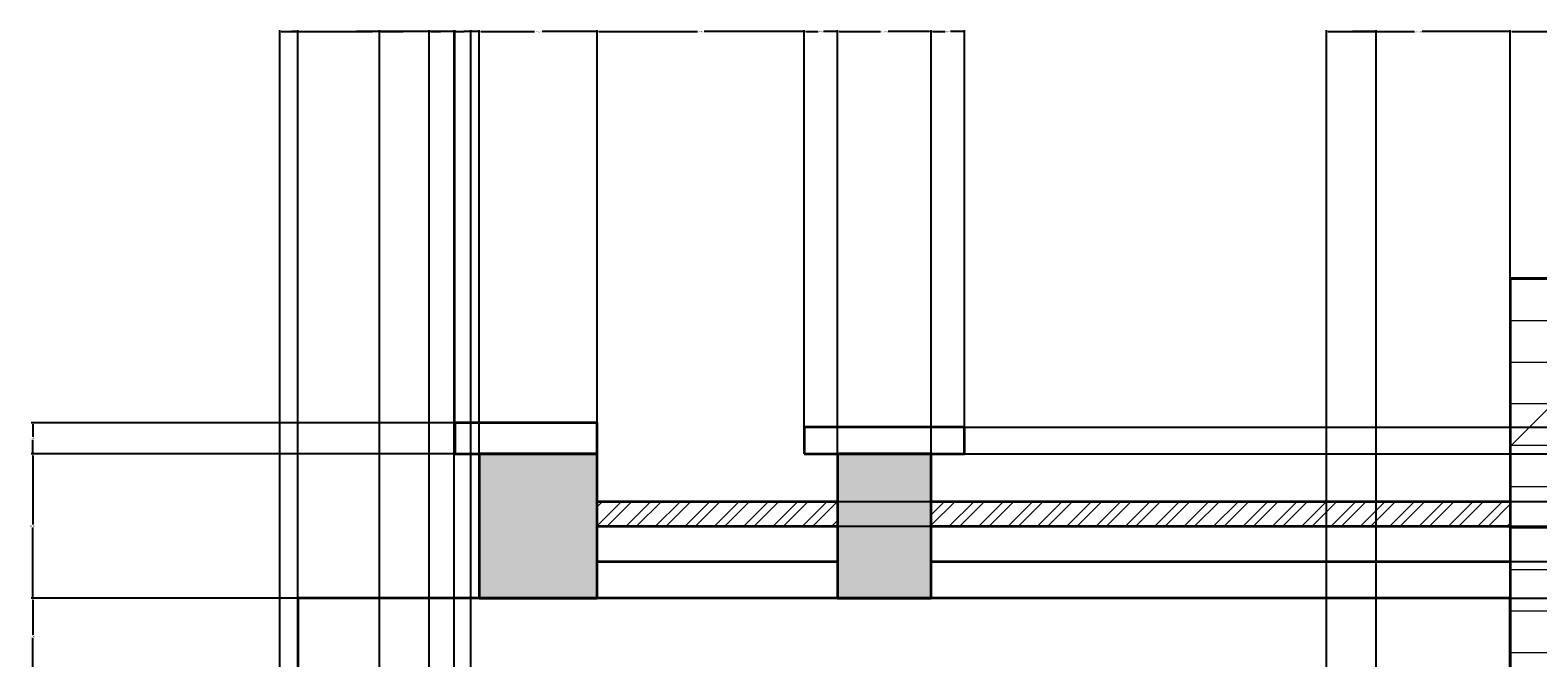
# Model space of a CAD drawing. Units: inches. Extents: x -13 to 630, y -103 to 275.
# Tile 5 of 9: x -13 to 168, y 199 to 275. Entities that reach past the tile are written whole.
import ezdxf

# ---------------------------------------------------------------- set-up
doc = ezdxf.new("R2010")
doc.units = ezdxf.units.IN
doc.header["$MEASUREMENT"] = 0
for name, color, linetype, lineweight in [('A-ANNO-DIMS', 2, 'Continuous', 18), ('A-ELEV', 7, 'Continuous', 35), ('A-ELEV-PATT', 8, 'Continuous', 13)]:
    doc.layers.add(name, color=color, linetype=linetype, lineweight=lineweight)
doc.styles.get("Standard").update_dxf_attribs({"font": 'arial.ttf'})
doc.dimstyles.get("Standard").update_dxf_attribs({"dimtxt": 0.18, "dimasz": 0.18, "dimexe": 0.18, "dimexo": 0.0625, "dimgap": 0.09, "dimtad": 0, "dimtih": 1, "dimtoh": 1, "dimdec": 4, "dimzin": 0, "dimdsep": 46, "dimtxsty": 'Standard', "dimcen": 0.09, "dimadec": 0, "dimazin": 0, "dimtfac": 1, "dimtdec": 4, "dimtofl": 0, "dimtmove": 0, "dimatfit": 3, "dimfxl": 1, "dimtolj": 1, "dimtzin": 0, "dimarcsym": 0})

# ---------------------------------------------------------------- blocks, each defined once
blk = doc.blocks.new('*D7')
at = {"layer": 'A-ANNO-DIMS', "color": 0, "lineweight": -2, "transparency": 16777216}
for p, q in [((16.71, 5.14), (16.71, 275.01)), ((16.89, 274.83), (25.5, 274.83)), ((34.53, 274.83), (25.92, 274.83)), ((34.71, 5.14), (34.71, 275.01))]:
    blk.add_line(p, q, dxfattribs=at)
at = {"layer": 'A-ANNO-DIMS', "color": 0, "transparency": 16777216}
for points in [[(16.89, 274.86), (16.89, 274.8), (16.71, 274.83)], [(34.53, 274.86), (34.53, 274.8), (34.71, 274.83)]]:
    blk.add_solid(points, dxfattribs=at)
at = {"layer": 'Defpoints', "color": 0, "transparency": 16777216}
for p in [(34.71, 274.83), (16.71, 5.08), (34.71, 5.08)]:
    blk.add_point(p, dxfattribs=at)
at = {"layer": 'A-ANNO-DIMS', "color": 0, "transparency": 16777216, "insert": (25.71, 274.83), "char_height": 0.18, "attachment_point": 5}
blk.add_mtext('\\A1;18', dxfattribs=at)
blk = doc.blocks.new('*D8')
at = {"layer": 'A-ANNO-DIMS', "color": 0, "lineweight": -2, "transparency": 16777216}
for p, q in [((142.71, 5.14), (142.71, 275.01)), ((142.89, 274.83), (153.31, 274.83)), ((164.66, 274.83), (154.24, 274.83)), ((164.84, 5.14), (164.84, 275.01))]:
    blk.add_line(p, q, dxfattribs=at)
at = {"layer": 'A-ANNO-DIMS', "color": 0, "transparency": 16777216}
for points in [[(142.89, 274.86), (142.89, 274.8), (142.71, 274.83)], [(164.66, 274.86), (164.66, 274.8), (164.84, 274.83)]]:
    blk.add_solid(points, dxfattribs=at)
at = {"layer": 'Defpoints', "color": 0, "transparency": 16777216}
for p in [(164.84, 274.83), (142.71, 5.08), (164.84, 5.08)]:
    blk.add_point(p, dxfattribs=at)
at = {"layer": 'A-ANNO-DIMS', "color": 0, "transparency": 16777216, "insert": (153.78, 274.83), "char_height": 0.18, "attachment_point": 5}
blk.add_mtext('\\A1;22.133', dxfattribs=at)
blk = doc.blocks.new('*D27')
at = {"layer": 'A-ANNO-DIMS', "color": 0, "lineweight": -2, "transparency": 16777216}
for p, q in [((164.84, 245.14), (164.84, 275.01)), ((165.02, 274.83), (254.62, 274.83)), ((345.13, 274.83), (255.53, 274.83)), ((345.31, 245.14), (345.31, 275.01))]:
    blk.add_line(p, q, dxfattribs=at)
at = {"layer": 'A-ANNO-DIMS', "color": 0, "transparency": 16777216}
for points in [[(165.02, 274.86), (165.02, 274.8), (164.84, 274.83)], [(345.13, 274.86), (345.13, 274.8), (345.31, 274.83)]]:
    blk.add_solid(points, dxfattribs=at)
at = {"layer": 'Defpoints', "color": 0, "transparency": 16777216}
for p in [(345.31, 274.83), (164.84, 245.08), (345.31, 245.08)]:
    blk.add_point(p, dxfattribs=at)
at = {"layer": 'A-ANNO-DIMS', "color": 0, "transparency": 16777216, "insert": (255.08, 274.83), "char_height": 0.18, "attachment_point": 5}
blk.add_mtext('\\A1;180.46', dxfattribs=at)
blk = doc.blocks.new('*D30')
at = {"layer": 'A-ANNO-DIMS', "color": 0, "lineweight": -2, "transparency": 16777216}
for p, q in [((164.84, 245.14), (164.84, 275.01)), ((165.02, 274.83), (170.63, 274.83)), ((176.66, 274.83), (171.05, 274.83)), ((176.84, 233.14), (176.84, 275.01))]:
    blk.add_line(p, q, dxfattribs=at)
at = {"layer": 'A-ANNO-DIMS', "color": 0, "transparency": 16777216}
for points in [[(165.02, 274.86), (165.02, 274.8), (164.84, 274.83)], [(176.66, 274.86), (176.66, 274.8), (176.84, 274.83)]]:
    blk.add_solid(points, dxfattribs=at)
at = {"layer": 'Defpoints', "color": 0, "transparency": 16777216}
for p in [(176.84, 274.83), (164.84, 245.08), (176.84, 233.08)]:
    blk.add_point(p, dxfattribs=at)
at = {"layer": 'A-ANNO-DIMS', "color": 0, "transparency": 16777216, "insert": (170.84, 274.83), "char_height": 0.18, "attachment_point": 5}
blk.add_mtext('\\A1;12', dxfattribs=at)
blk = doc.blocks.new('*D67')
at = {"layer": 'A-ANNO-DIMS', "color": 0, "lineweight": -2, "transparency": 16777216}
for p, q in [((28.71, 113.14), (28.71, 275.01)), ((28.89, 274.83), (31.56, 274.83)), ((34.53, 274.83), (31.86, 274.83)), ((34.71, 107.14), (34.71, 275.01))]:
    blk.add_line(p, q, dxfattribs=at)
at = {"layer": 'A-ANNO-DIMS', "color": 0, "transparency": 16777216}
for points in [[(28.89, 274.86), (28.89, 274.8), (28.71, 274.83)], [(34.53, 274.86), (34.53, 274.8), (34.71, 274.83)]]:
    blk.add_solid(points, dxfattribs=at)
at = {"layer": 'Defpoints', "color": 0, "transparency": 16777216}
for p in [(34.71, 274.83), (28.71, 113.08), (34.71, 107.08)]:
    blk.add_point(p, dxfattribs=at)
at = {"layer": 'A-ANNO-DIMS', "color": 0, "transparency": 16777216, "insert": (31.71, 274.83), "char_height": 0.18, "attachment_point": 5}
blk.add_mtext('\\A1;6', dxfattribs=at)
blk = doc.blocks.new('*D68')
at = {"layer": 'A-ANNO-DIMS', "color": 0, "lineweight": -2, "transparency": 16777216}
for p, q in [((34.71, 107.14), (34.71, 275.01)), ((34.89, 274.83), (36.06, 274.83)), ((37.53, 274.83), (36.36, 274.83)), ((37.71, 104.14), (37.71, 275.01))]:
    blk.add_line(p, q, dxfattribs=at)
at = {"layer": 'A-ANNO-DIMS', "color": 0, "transparency": 16777216}
for points in [[(34.89, 274.86), (34.89, 274.8), (34.71, 274.83)], [(37.53, 274.86), (37.53, 274.8), (37.71, 274.83)]]:
    blk.add_solid(points, dxfattribs=at)
at = {"layer": 'Defpoints', "color": 0, "transparency": 16777216}
for p in [(37.71, 274.83), (34.71, 107.08), (37.71, 104.08)]:
    blk.add_point(p, dxfattribs=at)
at = {"layer": 'A-ANNO-DIMS', "color": 0, "transparency": 16777216, "insert": (36.21, 274.83), "char_height": 0.18, "attachment_point": 5}
blk.add_mtext('\\A1;3', dxfattribs=at)
blk = doc.blocks.new('*D69')
at = {"layer": 'A-ANNO-DIMS', "color": 0, "lineweight": -2, "transparency": 16777216}
for p, q in [((37.71, 104.14), (37.71, 275.01)), ((37.89, 274.83), (38.56, 274.83)), ((39.53, 274.83), (38.86, 274.83)), ((39.71, 102.14), (39.71, 275.01))]:
    blk.add_line(p, q, dxfattribs=at)
at = {"layer": 'A-ANNO-DIMS', "color": 0, "transparency": 16777216}
for points in [[(37.89, 274.86), (37.89, 274.8), (37.71, 274.83)], [(39.53, 274.86), (39.53, 274.8), (39.71, 274.83)]]:
    blk.add_solid(points, dxfattribs=at)
at = {"layer": 'Defpoints', "color": 0, "transparency": 16777216}
for p in [(39.71, 274.83), (37.71, 104.08), (39.71, 102.08)]:
    blk.add_point(p, dxfattribs=at)
at = {"layer": 'A-ANNO-DIMS', "color": 0, "transparency": 16777216, "insert": (38.71, 274.83), "char_height": 0.18, "attachment_point": 5}
blk.add_mtext('\\A1;2', dxfattribs=at)
blk = doc.blocks.new('*D70')
at = {"layer": 'A-ANNO-DIMS', "color": 0, "lineweight": -2, "transparency": 16777216}
for p, q in [((142.71, 107.14), (142.71, 275.01)), ((142.89, 274.83), (145.56, 274.83)), ((148.53, 274.83), (145.86, 274.83)), ((148.71, 113.14), (148.71, 275.01))]:
    blk.add_line(p, q, dxfattribs=at)
at = {"layer": 'A-ANNO-DIMS', "color": 0, "transparency": 16777216}
for points in [[(142.89, 274.86), (142.89, 274.8), (142.71, 274.83)], [(148.53, 274.86), (148.53, 274.8), (148.71, 274.83)]]:
    blk.add_solid(points, dxfattribs=at)
at = {"layer": 'Defpoints', "color": 0, "transparency": 16777216}
for p in [(148.71, 274.83), (148.71, 113.08), (142.71, 107.08)]:
    blk.add_point(p, dxfattribs=at)
at = {"layer": 'A-ANNO-DIMS', "color": 0, "transparency": 16777216, "insert": (145.71, 274.83), "char_height": 0.18, "attachment_point": 5}
blk.add_mtext('\\A1;6', dxfattribs=at)
blk = doc.blocks.new('*D88')
at = {"layer": 'A-ANNO-DIMS', "color": 0, "lineweight": -2, "transparency": 16777216}
for p, q in [((18.81, 206.53), (-13.22, 206.53)), ((-13.04, 206.35), (-13.04, 202.11)), ((-13.04, 197.5), (-13.04, 201.74)), ((18.81, 197.32), (-13.22, 197.32))]:
    blk.add_line(p, q, dxfattribs=at)
at = {"layer": 'A-ANNO-DIMS', "color": 0, "transparency": 16777216}
for points in [[(-13.07, 206.35), (-13.01, 206.35), (-13.04, 206.53)], [(-13.07, 197.5), (-13.01, 197.5), (-13.04, 197.32)]]:
    blk.add_solid(points, dxfattribs=at)
at = {"layer": 'Defpoints', "color": 0, "transparency": 16777216}
for p in [(-13.04, 206.53), (18.87, 206.53), (18.87, 197.32)]:
    blk.add_point(p, dxfattribs=at)
at = {"layer": 'A-ANNO-DIMS', "color": 0, "transparency": 16777216, "insert": (-13.04, 201.92), "char_height": 0.18, "attachment_point": 5}
blk.add_mtext('\\A1;9.206', dxfattribs=at)
blk = doc.blocks.new('*D89')
at = {"layer": 'A-ANNO-DIMS', "color": 0, "lineweight": -2, "transparency": 16777216}
for p, q in [((95.18, 210.97), (630.03, 210.97)), ((629.85, 210.79), (629.85, 208.93)), ((629.85, 206.71), (629.85, 208.57)), ((95.18, 206.53), (630.03, 206.53))]:
    blk.add_line(p, q, dxfattribs=at)
at = {"layer": 'A-ANNO-DIMS', "color": 0, "transparency": 16777216}
for points in [[(629.82, 210.79), (629.88, 210.79), (629.85, 210.97)], [(629.82, 206.71), (629.88, 206.71), (629.85, 206.53)]]:
    blk.add_solid(points, dxfattribs=at)
at = {"layer": 'Defpoints', "color": 0, "transparency": 16777216}
for p in [(95.12, 210.97), (629.85, 210.97), (95.12, 206.53)]:
    blk.add_point(p, dxfattribs=at)
at = {"layer": 'A-ANNO-DIMS', "color": 0, "transparency": 16777216, "insert": (629.85, 208.75), "char_height": 0.18, "attachment_point": 5}
blk.add_mtext('\\A1;4.442', dxfattribs=at)
blk = doc.blocks.new('*D90')
at = {"layer": 'A-ANNO-DIMS', "color": 0, "lineweight": -2, "transparency": 16777216}
for p, q in [((95.18, 218.21), (630.03, 218.21)), ((629.85, 218.03), (629.85, 214.77)), ((629.85, 211.15), (629.85, 214.41)), ((95.18, 210.97), (630.03, 210.97))]:
    blk.add_line(p, q, dxfattribs=at)
at = {"layer": 'A-ANNO-DIMS', "color": 0, "transparency": 16777216}
for points in [[(629.82, 218.03), (629.88, 218.03), (629.85, 218.21)], [(629.82, 211.15), (629.88, 211.15), (629.85, 210.97)]]:
    blk.add_solid(points, dxfattribs=at)
at = {"layer": 'Defpoints', "color": 0, "transparency": 16777216}
for p in [(95.12, 218.21), (629.85, 218.21), (95.12, 210.97)]:
    blk.add_point(p, dxfattribs=at)
at = {"layer": 'A-ANNO-DIMS', "color": 0, "transparency": 16777216, "insert": (629.85, 214.59), "char_height": 0.18, "attachment_point": 5}
blk.add_mtext('\\A1;7.236', dxfattribs=at)
blk = doc.blocks.new('*D91')
at = {"layer": 'A-ANNO-DIMS', "color": 0, "lineweight": -2, "transparency": 16777216}
for p, q in [((54.98, 218.21), (630.03, 218.21)), ((629.85, 218.03), (629.85, 216.9)), ((629.85, 215.41), (629.85, 216.54)), ((54.98, 215.23), (630.03, 215.23))]:
    blk.add_line(p, q, dxfattribs=at)
at = {"layer": 'A-ANNO-DIMS', "color": 0, "transparency": 16777216}
for points in [[(629.82, 218.03), (629.88, 218.03), (629.85, 218.21)], [(629.82, 215.41), (629.88, 215.41), (629.85, 215.23)]]:
    blk.add_solid(points, dxfattribs=at)
at = {"layer": 'Defpoints', "color": 0, "transparency": 16777216}
for p in [(54.92, 218.21), (629.85, 218.21), (54.92, 215.23)]:
    blk.add_point(p, dxfattribs=at)
at = {"layer": 'A-ANNO-DIMS', "color": 0, "transparency": 16777216, "insert": (629.85, 216.72), "char_height": 0.18, "attachment_point": 5}
blk.add_mtext('\\A1;2.972', dxfattribs=at)
blk = doc.blocks.new('*D92')
at = {"layer": 'A-ANNO-DIMS', "color": 0, "lineweight": -2, "transparency": 16777216}
for p, q in [((40.66, 223.94), (-13.22, 223.94)), ((-13.04, 223.76), (-13.04, 215.41)), ((-13.04, 206.71), (-13.04, 215.05)), ((40.66, 206.53), (-13.22, 206.53))]:
    blk.add_line(p, q, dxfattribs=at)
at = {"layer": 'A-ANNO-DIMS', "color": 0, "transparency": 16777216}
for points in [[(-13.07, 223.76), (-13.01, 223.76), (-13.04, 223.94)], [(-13.07, 206.71), (-13.01, 206.71), (-13.04, 206.53)]]:
    blk.add_solid(points, dxfattribs=at)
at = {"layer": 'Defpoints', "color": 0, "transparency": 16777216}
for p in [(-13.04, 223.94), (40.72, 223.94), (40.72, 206.53)]:
    blk.add_point(p, dxfattribs=at)
at = {"layer": 'A-ANNO-DIMS', "color": 0, "transparency": 16777216, "insert": (-13.04, 215.23), "char_height": 0.18, "attachment_point": 5}
blk.add_mtext('\\A1;17.41', dxfattribs=at)
blk = doc.blocks.new('*D93')
at = {"layer": 'A-ANNO-DIMS', "color": 0, "lineweight": -2, "transparency": 16777216}
for p, q in [((37.71, 227.69), (-13.22, 227.69)), ((-13.04, 227.51), (-13.04, 226)), ((-13.04, 224.12), (-13.04, 225.63)), ((37.71, 223.94), (-13.22, 223.94))]:
    blk.add_line(p, q, dxfattribs=at)
at = {"layer": 'A-ANNO-DIMS', "color": 0, "transparency": 16777216}
for points in [[(-13.07, 227.51), (-13.01, 227.51), (-13.04, 227.69)], [(-13.07, 224.12), (-13.01, 224.12), (-13.04, 223.94)]]:
    blk.add_solid(points, dxfattribs=at)
at = {"layer": 'Defpoints', "color": 0, "transparency": 16777216}
for p in [(-13.04, 227.69), (37.77, 227.69), (37.77, 223.94)]:
    blk.add_point(p, dxfattribs=at)
at = {"layer": 'A-ANNO-DIMS', "color": 0, "transparency": 16777216, "insert": (-13.04, 225.81), "char_height": 0.18, "attachment_point": 5}
blk.add_mtext('\\A1;3.748', dxfattribs=at)
blk = doc.blocks.new('*D94')
at = {"layer": 'A-ANNO-DIMS', "color": 0, "lineweight": -2, "transparency": 16777216}
for p, q in [((99.2, 227.15), (630.03, 227.15)), ((629.85, 226.97), (629.85, 225.73)), ((629.85, 224.12), (629.85, 225.36)), ((99.2, 223.94), (630.03, 223.94))]:
    blk.add_line(p, q, dxfattribs=at)
at = {"layer": 'A-ANNO-DIMS', "color": 0, "transparency": 16777216}
for points in [[(629.82, 226.97), (629.88, 226.97), (629.85, 227.15)], [(629.82, 224.12), (629.88, 224.12), (629.85, 223.94)]]:
    blk.add_solid(points, dxfattribs=at)
at = {"layer": 'Defpoints', "color": 0, "transparency": 16777216}
for p in [(99.14, 227.15), (629.85, 227.15), (99.14, 223.94)]:
    blk.add_point(p, dxfattribs=at)
at = {"layer": 'A-ANNO-DIMS', "color": 0, "transparency": 16777216, "insert": (629.85, 225.55), "char_height": 0.18, "attachment_point": 5}
blk.add_mtext('\\A1;3.21', dxfattribs=at)
blk = doc.blocks.new('*D95')
at = {"layer": 'A-ANNO-DIMS', "color": 0, "lineweight": -2, "transparency": 16777216}
for p, q in [((16.71, 125.14), (16.71, 275.01)), ((16.89, 274.83), (17.47, 274.83)), ((18.69, 274.83), (18.12, 274.83)), ((18.87, 206.59), (18.87, 275.01))]:
    blk.add_line(p, q, dxfattribs=at)
at = {"layer": 'A-ANNO-DIMS', "color": 0, "transparency": 16777216}
for points in [[(16.89, 274.86), (16.89, 274.8), (16.71, 274.83)], [(18.69, 274.86), (18.69, 274.8), (18.87, 274.83)]]:
    blk.add_solid(points, dxfattribs=at)
at = {"layer": 'Defpoints', "color": 0, "transparency": 16777216}
for p in [(18.87, 274.83), (18.87, 206.53), (16.71, 125.08)]:
    blk.add_point(p, dxfattribs=at)
at = {"layer": 'A-ANNO-DIMS', "color": 0, "transparency": 16777216, "insert": (17.79, 274.83), "char_height": 0.18, "attachment_point": 5}
blk.add_mtext('\\A1;2.16', dxfattribs=at)
blk = doc.blocks.new('*D96')
at = {"layer": 'A-ANNO-DIMS', "color": 0, "lineweight": -2, "transparency": 16777216}
for p, q in [((18.87, 206.59), (18.87, 275.01)), ((19.05, 274.83), (27.87, 274.83)), ((37.59, 274.83), (28.78, 274.83)), ((37.77, 227.75), (37.77, 275.01))]:
    blk.add_line(p, q, dxfattribs=at)
at = {"layer": 'A-ANNO-DIMS', "color": 0, "transparency": 16777216}
for points in [[(19.05, 274.86), (19.05, 274.8), (18.87, 274.83)], [(37.59, 274.86), (37.59, 274.8), (37.77, 274.83)]]:
    blk.add_solid(points, dxfattribs=at)
at = {"layer": 'Defpoints', "color": 0, "transparency": 16777216}
for p in [(37.77, 274.83), (37.77, 227.69), (18.87, 206.53)]:
    blk.add_point(p, dxfattribs=at)
at = {"layer": 'A-ANNO-DIMS', "color": 0, "transparency": 16777216, "insert": (28.32, 274.83), "char_height": 0.18, "attachment_point": 5}
blk.add_mtext('\\A1;18.898', dxfattribs=at)
blk = doc.blocks.new('*D97')
at = {"layer": 'A-ANNO-DIMS', "color": 0, "lineweight": -2, "transparency": 16777216}
for p, q in [((37.77, 227.75), (37.77, 275.01)), ((37.95, 274.83), (38.92, 274.83)), ((40.54, 274.83), (39.57, 274.83)), ((40.72, 224), (40.72, 275.01))]:
    blk.add_line(p, q, dxfattribs=at)
at = {"layer": 'A-ANNO-DIMS', "color": 0, "transparency": 16777216}
for points in [[(37.95, 274.86), (37.95, 274.8), (37.77, 274.83)], [(40.54, 274.86), (40.54, 274.8), (40.72, 274.83)]]:
    blk.add_solid(points, dxfattribs=at)
at = {"layer": 'Defpoints', "color": 0, "transparency": 16777216}
for p in [(40.72, 274.83), (37.77, 227.69), (40.72, 223.94)]:
    blk.add_point(p, dxfattribs=at)
at = {"layer": 'A-ANNO-DIMS', "color": 0, "transparency": 16777216, "insert": (39.24, 274.83), "char_height": 0.18, "attachment_point": 5}
blk.add_mtext('\\A1;2.95', dxfattribs=at)
blk = doc.blocks.new('*D98')
at = {"layer": 'A-ANNO-DIMS', "color": 0, "lineweight": -2, "transparency": 16777216}
for p, q in [((40.72, 224), (40.72, 275.01)), ((40.9, 274.83), (47.36, 274.83)), ((54.74, 274.83), (48.28, 274.83)), ((54.92, 224), (54.92, 275.01))]:
    blk.add_line(p, q, dxfattribs=at)
at = {"layer": 'A-ANNO-DIMS', "color": 0, "transparency": 16777216}
for points in [[(40.9, 274.86), (40.9, 274.8), (40.72, 274.83)], [(54.74, 274.86), (54.74, 274.8), (54.92, 274.83)]]:
    blk.add_solid(points, dxfattribs=at)
at = {"layer": 'Defpoints', "color": 0, "transparency": 16777216}
for p in [(54.92, 274.83), (40.72, 223.94), (54.92, 223.94)]:
    blk.add_point(p, dxfattribs=at)
at = {"layer": 'A-ANNO-DIMS', "color": 0, "transparency": 16777216, "insert": (47.82, 274.83), "char_height": 0.18, "attachment_point": 5}
blk.add_mtext('\\A1;14.203', dxfattribs=at)
blk = doc.blocks.new('*D99')
at = {"layer": 'A-ANNO-DIMS', "color": 0, "lineweight": -2, "transparency": 16777216}
for p, q in [((54.92, 224), (54.92, 275.01)), ((55.1, 274.83), (66.99, 274.83)), ((79.66, 274.83), (67.78, 274.83)), ((79.84, 227.21), (79.84, 275.01))]:
    blk.add_line(p, q, dxfattribs=at)
at = {"layer": 'A-ANNO-DIMS', "color": 0, "transparency": 16777216}
for points in [[(55.1, 274.86), (55.1, 274.8), (54.92, 274.83)], [(79.66, 274.86), (79.66, 274.8), (79.84, 274.83)]]:
    blk.add_solid(points, dxfattribs=at)
at = {"layer": 'Defpoints', "color": 0, "transparency": 16777216}
for p in [(79.84, 274.83), (79.84, 227.15), (54.92, 223.94)]:
    blk.add_point(p, dxfattribs=at)
at = {"layer": 'A-ANNO-DIMS', "color": 0, "transparency": 16777216, "insert": (67.38, 274.83), "char_height": 0.18, "attachment_point": 5}
blk.add_mtext('\\A1;24.92', dxfattribs=at)
blk = doc.blocks.new('*D100')
at = {"layer": 'A-ANNO-DIMS', "color": 0, "lineweight": -2, "transparency": 16777216}
for p, q in [((79.84, 227.21), (79.84, 275.01)), ((80.02, 274.83), (81.53, 274.83)), ((83.68, 274.83), (82.18, 274.83)), ((83.86, 224), (83.86, 275.01))]:
    blk.add_line(p, q, dxfattribs=at)
at = {"layer": 'A-ANNO-DIMS', "color": 0, "transparency": 16777216}
for points in [[(80.02, 274.86), (80.02, 274.8), (79.84, 274.83)], [(83.68, 274.86), (83.68, 274.8), (83.86, 274.83)]]:
    blk.add_solid(points, dxfattribs=at)
at = {"layer": 'Defpoints', "color": 0, "transparency": 16777216}
for p in [(83.86, 274.83), (79.84, 227.15), (83.86, 223.94)]:
    blk.add_point(p, dxfattribs=at)
at = {"layer": 'A-ANNO-DIMS', "color": 0, "transparency": 16777216, "insert": (81.85, 274.83), "char_height": 0.18, "attachment_point": 5}
blk.add_mtext('\\A1;4.02', dxfattribs=at)
blk = doc.blocks.new('*D101')
at = {"layer": 'A-ANNO-DIMS', "color": 0, "lineweight": -2, "transparency": 16777216}
for p, q in [((83.86, 224), (83.86, 275.01)), ((84.04, 274.83), (89.03, 274.83)), ((94.94, 274.83), (89.95, 274.83)), ((95.12, 224), (95.12, 275.01))]:
    blk.add_line(p, q, dxfattribs=at)
at = {"layer": 'A-ANNO-DIMS', "color": 0, "transparency": 16777216}
for points in [[(84.04, 274.86), (84.04, 274.8), (83.86, 274.83)], [(94.94, 274.86), (94.94, 274.8), (95.12, 274.83)]]:
    blk.add_solid(points, dxfattribs=at)
at = {"layer": 'Defpoints', "color": 0, "transparency": 16777216}
for p in [(95.12, 274.83), (83.86, 223.94), (95.12, 223.94)]:
    blk.add_point(p, dxfattribs=at)
at = {"layer": 'A-ANNO-DIMS', "color": 0, "transparency": 16777216, "insert": (89.49, 274.83), "char_height": 0.18, "attachment_point": 5}
blk.add_mtext('\\A1;11.255', dxfattribs=at)
blk = doc.blocks.new('*D102')
at = {"layer": 'A-ANNO-DIMS', "color": 0, "lineweight": -2, "transparency": 16777216}
for p, q in [((95.12, 224), (95.12, 275.01)), ((95.3, 274.83), (96.8, 274.83)), ((98.96, 274.83), (97.45, 274.83)), ((99.14, 227.21), (99.14, 275.01))]:
    blk.add_line(p, q, dxfattribs=at)
at = {"layer": 'A-ANNO-DIMS', "color": 0, "transparency": 16777216}
for points in [[(95.3, 274.86), (95.3, 274.8), (95.12, 274.83)], [(98.96, 274.86), (98.96, 274.8), (99.14, 274.83)]]:
    blk.add_solid(points, dxfattribs=at)
at = {"layer": 'Defpoints', "color": 0, "transparency": 16777216}
for p in [(99.14, 274.83), (99.14, 227.15), (95.12, 223.94)]:
    blk.add_point(p, dxfattribs=at)
at = {"layer": 'A-ANNO-DIMS', "color": 0, "transparency": 16777216, "insert": (97.13, 274.83), "char_height": 0.18, "attachment_point": 5}
blk.add_mtext('\\A1;4.02', dxfattribs=at)

msp = doc.modelspace()

# ---------------------------------------------------------------- hatches: boundary and pattern name
at = {"layer": 'A-ELEV-PATT', "transparency": 33554541}
h = msp.add_hatch(dxfattribs=at)
h.set_pattern_fill('DOLMIT', color=256, scale=20)
h.paths.add_polyline_path([(345.3061, 245.0808), (164.8443, 245.0808), (164.8443, 5.0808), (176.8443, 5.0808), (176.8443, 233.0808), (333.3061, 233.0808), (333.3061, 5.0808), (345.3061, 5.0808)])
at = {"layer": 'A-ELEV-PATT'}
h = msp.add_hatch(dxfattribs=at)
h.set_pattern_fill('BRSTONE', color=256, scale=20)
h.paths.add_polyline_path([(120.6641, 172.7854), (64.9953, 172.7854, 0.41421356), (54.9953, 162.7854), (54.9953, 125.0808), (59.9953, 125.0808), (59.9953, 162.7854, -0.41421356), (64.9953, 167.7854), (120.6641, 167.7854, -0.41421356), (125.6641, 162.7854), (125.6641, 125.0808), (130.6641, 125.0808), (130.6641, 162.7854, 0.41421356)])
h.paths.add_polyline_path([(439.5513, 172.7854), (383.8825, 172.7854, 0.41421356), (373.8825, 162.7854), (373.8825, 125.0808), (378.8825, 125.0808), (378.8825, 162.7854, -0.41421356), (383.8825, 167.7854), (439.5513, 167.7854, -0.41421356), (444.5513, 162.7854), (444.5513, 125.0808), (449.5513, 125.0808), (449.5513, 162.7854, 0.41421356)])
h.paths.add_polyline_path([(364.7117, 113.0808), (484.7117, 113.0808), (484.7117, 5.0808), (496.7117, 5.0808), (496.7117, 125.0808), (345.3061, 125.0808), (345.3061, 5.0808), (364.7117, 5.0808)])
h.paths.add_polyline_path([(164.8443, 125.0808), (28.7117, 125.0808), (16.7117, 125.0808), (16.7117, 5.0808), (28.7117, 5.0808), (28.7117, 113.0808), (148.7117, 113.0808), (148.7117, 5.0808), (164.8443, 5.0808)])
h.paths.add_polyline_path([(95.1171, 223.9392), (83.8622, 223.9392), (83.8622, 206.5279), (95.1171, 206.5279)])
h.paths.add_polyline_path([(54.9212, 223.9392), (40.7186, 223.9392), (40.7186, 206.5279), (54.9212, 206.5279)])
h.paths.add_polyline_path([(463.828, 223.9392), (449.6254, 223.9392), (449.6254, 206.5279), (463.828, 206.5279)])
h.paths.add_polyline_path([(420.6843, 223.9392), (409.4295, 223.9392), (409.4295, 206.5279), (420.6843, 206.5279)])
h = msp.add_hatch(dxfattribs=at)
h.set_pattern_fill('STEEL', color=256, scale=20)
h.set_pattern_definition([(45, (0, 0), (-1.767767, 1.767767), []), (45, (0, 1.25), (-1.767767, 1.767767), [])])
h.paths.add_polyline_path([(164.8443, 218.2056), (95.1171, 218.2056), (95.1171, 215.2335), (164.8443, 215.2335)])
h.paths.add_polyline_path([(83.8622, 218.2056), (54.9212, 218.2056), (54.9212, 215.2335), (83.8622, 215.2335)])
h.paths.add_polyline_path([(409.4295, 218.2056), (345.3061, 218.2056), (345.3061, 215.2335), (409.4295, 215.2335)])
h.paths.add_polyline_path([(449.6254, 218.2056), (420.6843, 218.2056), (420.6843, 215.2335), (449.6254, 215.2335)])
h.paths.add_polyline_path([(302.5258, 203.9359), (202.0208, 203.9359), (202.0208, 128.6551, -0.36718729), (252.2733, 187.858, -0.36718729), (302.5258, 128.6551)])

# ---------------------------------------------------------------- linework, layer by layer
at = {"layer": 'A-ELEV'}
for p, q in [((54.9212, 218.2056), (83.8622, 218.2056)), ((95.1171, 218.2056), (164.8443, 218.2056)), ((54.9212, 215.2335), (83.8622, 215.2335)), ((95.1171, 215.2335), (164.8443, 215.2335)), ((54.9212, 210.9698), (83.8622, 210.9698)), ((95.1171, 210.9698), (164.8443, 210.9698))]:
    msp.add_line(p, q, dxfattribs=at)
msp.add_lwpolyline([(345.3061, 5.0808), (345.3061, 245.0808), (164.8443, 245.0808), (164.8443, 5.0808)], dxfattribs=at)
for points in [[(37.7709, 223.9392), (54.9212, 223.9392), (54.9212, 227.6872), (37.7709, 227.6872)], [(79.8426, 223.9392), (99.1367, 223.9392), (99.1367, 227.1518), (79.8426, 227.1518)], [(40.7186, 206.5279), (54.9212, 206.5279), (54.9212, 223.9392), (40.7186, 223.9392)], [(83.8622, 206.5279), (95.1171, 206.5279), (95.1171, 223.9392), (83.8622, 223.9392)], [(18.8732, 197.3216), (164.8443, 197.3216), (164.8443, 206.5279), (18.8732, 206.5279)]]:
    msp.add_lwpolyline(points, close=True, dxfattribs=at)

# ---------------------------------------------------------------- dimensions: what is measured, and where the dimension line sits
at = {"layer": 'A-ANNO-DIMS'}
for base, p1, p2, override, picture, middle in [((34.7117, 274.8308), (16.7117, 5.0808), (34.7117, 5.0808), {"dimdec": 0, "dimlfac": 1, "dimrnd": 0, "dimzin": 0, "dimdsep": 46, "dimlunit": 2}, '*D7', (25.7117, 274.8308)), ((18.8732, 274.8308), (16.7117, 125.0808), (18.8732, 206.5279), {"dimdec": 2, "dimlfac": 1, "dimrnd": 0, "dimzin": 0, "dimdsep": 46, "dimlunit": 2}, '*D95', (17.7925, 274.8308)), ((37.7709, 274.8308), (18.8732, 206.5279), (37.7709, 227.6872), {"dimdec": 3, "dimlfac": 1, "dimrnd": 0, "dimzin": 0, "dimdsep": 46, "dimlunit": 2}, '*D96', (28.3221, 274.8308)), ((34.7117, 274.8308), (28.7117, 113.0808), (34.7117, 107.0808), {"dimdec": 0, "dimlfac": 1, "dimrnd": 0, "dimzin": 0, "dimdsep": 46, "dimlunit": 2}, '*D67', (31.7117, 274.8308)), ((37.7117, 274.8308), (34.7117, 107.0808), (37.7117, 104.0808), {"dimdec": 0, "dimlfac": 1, "dimrnd": 0, "dimzin": 0, "dimdsep": 46, "dimlunit": 2}, '*D68', (36.2117, 274.8308)), ((39.7117, 274.8308), (37.7117, 104.0808), (39.7117, 102.0808), {"dimdec": 0, "dimlfac": 1, "dimrnd": 0, "dimzin": 0, "dimdsep": 46, "dimlunit": 2}, '*D69', (38.7117, 274.8308)), ((40.7186, 274.8308), (37.7709, 227.6872), (40.7186, 223.9392), {"dimdec": 2, "dimlfac": 1, "dimrnd": 0, "dimzin": 0, "dimdsep": 46, "dimlunit": 2}, '*D97', (39.2448, 274.8308)), ((54.9212, 274.8308), (40.7186, 223.9392), (54.9212, 223.9392), {"dimdec": 3, "dimlfac": 1, "dimrnd": 0, "dimzin": 0, "dimdsep": 46, "dimlunit": 2}, '*D98', (47.8199, 274.8308)), ((79.8426, 274.8308), (54.9212, 223.9392), (79.8426, 227.1518), {"dimdec": 2, "dimlfac": 1, "dimrnd": 0, "dimzin": 0, "dimdsep": 46, "dimlunit": 2}, '*D99', (67.3819, 274.8308)), ((83.8622, 274.8308), (79.8426, 227.1518), (83.8622, 223.9392), {"dimdec": 2, "dimlfac": 1, "dimrnd": 0, "dimzin": 0, "dimdsep": 46, "dimlunit": 2}, '*D100', (81.8524, 274.8308)), ((95.1171, 274.8308), (83.8622, 223.9392), (95.1171, 223.9392), {"dimdec": 3, "dimlfac": 1, "dimrnd": 0, "dimzin": 0, "dimdsep": 46, "dimlunit": 2}, '*D101', (89.4896, 274.8308)), ((99.1367, 274.8308), (95.1171, 223.9392), (99.1367, 227.1518), {"dimdec": 2, "dimlfac": 1, "dimrnd": 0, "dimzin": 0, "dimdsep": 46, "dimlunit": 2}, '*D102', (97.1269, 274.8308)), ((164.8443, 274.8308), (142.7117, 5.0808), (164.8443, 5.0808), {"dimdec": 3, "dimlfac": 1, "dimrnd": 0, "dimzin": 0, "dimdsep": 46, "dimlunit": 2}, '*D8', (153.778, 274.8308)), ((148.7117, 274.8308), (142.7117, 107.0808), (148.7117, 113.0808), {"dimdec": 0, "dimlfac": 1, "dimrnd": 0, "dimzin": 0, "dimdsep": 46, "dimlunit": 2}, '*D70', (145.7117, 274.8308)), ((345.3061, 274.8308), (164.8443, 245.0808), (345.3061, 245.0808), {"dimdec": 2, "dimlfac": 1, "dimrnd": 0, "dimzin": 0, "dimdsep": 46, "dimlunit": 2}, '*D27', (255.0752, 274.8308)), ((176.8443, 274.8308), (164.8443, 245.0808), (176.8443, 233.0808), {"dimdec": 0, "dimlfac": 1, "dimrnd": 0, "dimzin": 0, "dimdsep": 46, "dimlunit": 2}, '*D30', (170.8443, 274.8308))]:
    dim = msp.add_linear_dim(base=base, p1=p1, p2=p2, dimstyle='Standard', override=override, dxfattribs=at)
    dim.commit()
    dim.dimension.update_dxf_attribs({"geometry": picture, "text_midpoint": middle})
for base, p1, p2, override, picture, middle in [((-13.0383, 227.6872), (37.7709, 223.9392), (37.7709, 227.6872), {"dimdec": 3, "dimlfac": 1, "dimrnd": 0, "dimzin": 0, "dimdsep": 46, "dimlunit": 2}, '*D93', (-13.0383, 225.8132)), ((629.8508, 227.1518), (99.1367, 223.9392), (99.1367, 227.1518), {"dimdec": 2, "dimlfac": 1, "dimrnd": 0, "dimzin": 0, "dimdsep": 46, "dimlunit": 2}, '*D94', (629.8508, 225.5455)), ((-13.0383, 223.9392), (40.7186, 206.5279), (40.7186, 223.9392), {"dimdec": 2, "dimlfac": 1, "dimrnd": 0, "dimzin": 0, "dimdsep": 46, "dimlunit": 2}, '*D92', (-13.0383, 215.2335)), ((629.8508, 218.2056), (54.9212, 215.2335), (54.9212, 218.2056), {"dimdec": 3, "dimlfac": 1, "dimrnd": 0, "dimzin": 0, "dimdsep": 46, "dimlunit": 2}, '*D91', (629.8508, 216.7196)), ((629.8508, 218.2056), (95.1171, 210.9698), (95.1171, 218.2056), {"dimdec": 3, "dimlfac": 1, "dimrnd": 0, "dimzin": 0, "dimdsep": 46, "dimlunit": 2}, '*D90', (629.8508, 214.5877)), ((629.8508, 210.9698), (95.1171, 206.5279), (95.1171, 210.9698), {"dimdec": 3, "dimlfac": 1, "dimrnd": 0, "dimzin": 0, "dimdsep": 46, "dimlunit": 2}, '*D89', (629.8508, 208.7489)), ((-13.0383, 206.5279), (18.8732, 197.3216), (18.8732, 206.5279), {"dimdec": 3, "dimlfac": 1, "dimrnd": 0, "dimzin": 0, "dimdsep": 46, "dimlunit": 2}, '*D88', (-13.0383, 201.9247))]:
    dim = msp.add_linear_dim(base=base, p1=p1, p2=p2, angle=90, dimstyle='Standard', override=override, dxfattribs=at)
    dim.commit()
    dim.dimension.update_dxf_attribs({"geometry": picture, "text_midpoint": middle})

doc.saveas('drawing.dxf')
